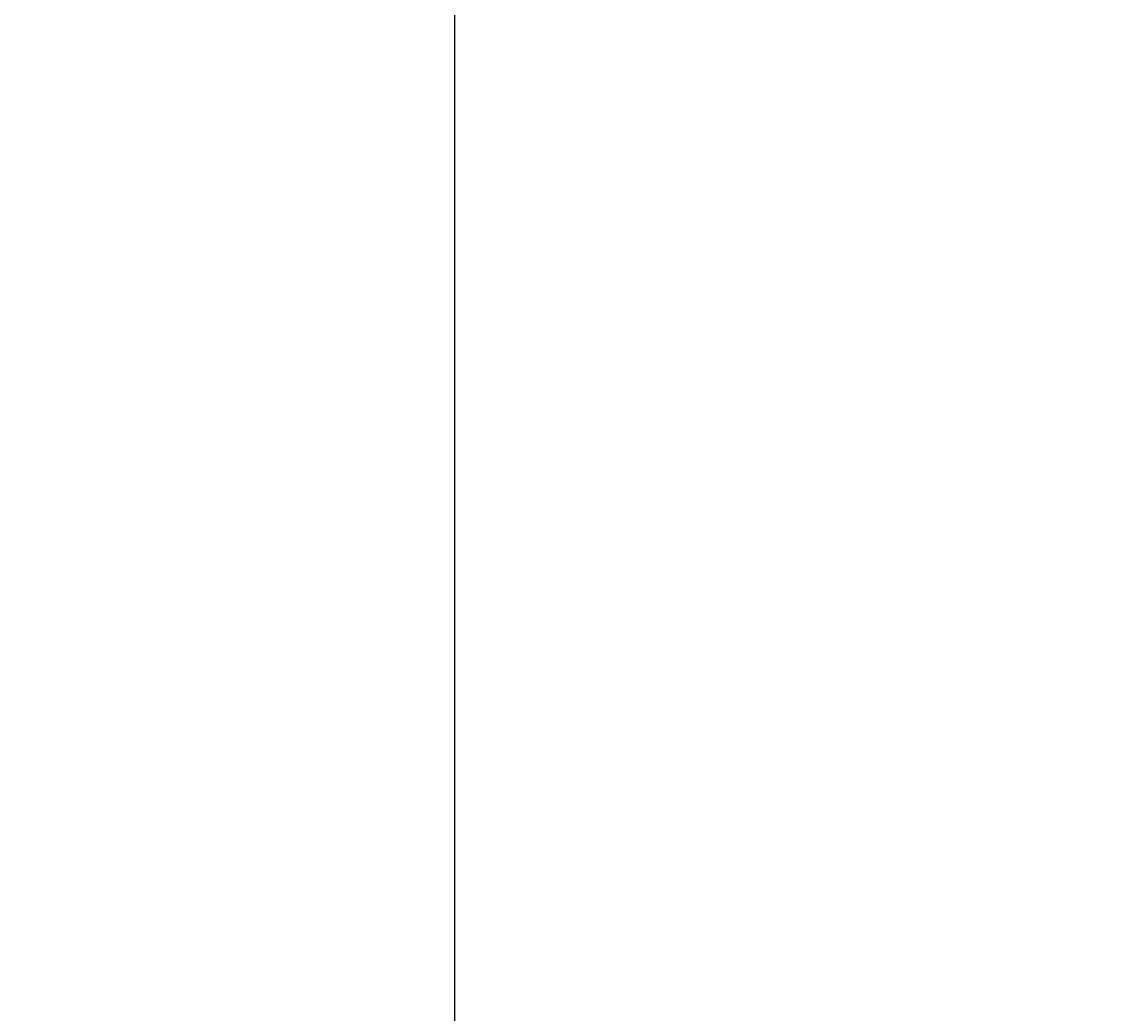
# Model space of a CAD drawing. Units: inches. Extents: x 1998 to 2588, y 1139 to 1977.
# Tile 83 of 134: x 2397 to 2425, y 1427 to 1452. Entities that reach past the tile are written whole.
import ezdxf

# ---------------------------------------------------------------- set-up
doc = ezdxf.new("R2010")
doc.units = ezdxf.units.IN
doc.layers.add('A-ANNO-DIMS', color=2, linetype='Continuous', lineweight=18)
doc.styles.get("Standard").update_dxf_attribs({"font": 'arial.ttf'})
doc.dimstyles.get("Standard").update_dxf_attribs({"dimtxt": 0.18, "dimasz": 0.18, "dimexe": 0.18, "dimexo": 0.0625, "dimgap": 0.09, "dimtad": 0, "dimtih": 1, "dimtoh": 1, "dimdec": 4, "dimzin": 0, "dimdsep": 46, "dimtxsty": 'Standard', "dimcen": 0.09, "dimadec": 0, "dimazin": 0, "dimtfac": 1, "dimtdec": 4, "dimtofl": 0, "dimtmove": 0, "dimatfit": 3, "dimfxl": 1, "dimtolj": 1, "dimtzin": 0, "dimarcsym": 0})

# ---------------------------------------------------------------- blocks, each defined once
blk = doc.blocks.new('*D23')
at = {"layer": 'A-ANNO-DIMS', "color": 0, "lineweight": -2, "transparency": 16777216}
for p, q in [((2549.179, 1476.17), (2549.179, 1138.602)), ((2059.473, 1413.17), (2059.473, 1138.602)), ((2059.653, 1138.782), (2303.928, 1138.782)), ((2548.999, 1138.782), (2304.723, 1138.782))]:
    blk.add_line(p, q, dxfattribs=at)
at = {"layer": 'A-ANNO-DIMS', "color": 0, "transparency": 16777216}
for points in [[(2059.653, 1138.812), (2059.653, 1138.752), (2059.473, 1138.782)], [(2548.999, 1138.812), (2548.999, 1138.752), (2549.179, 1138.782)]]:
    blk.add_solid(points, dxfattribs=at)
at = {"layer": 'Defpoints', "color": 0, "transparency": 16777216}
for p in [(2549.179, 1476.232), (2059.473, 1413.232), (2549.179, 1138.782)]:
    blk.add_point(p, dxfattribs=at)
at = {"layer": 'A-ANNO-DIMS', "color": 0, "transparency": 16777216, "insert": (2304.326, 1138.782), "char_height": 0.18, "attachment_point": 5}
blk.add_mtext('\\A1;489.7', dxfattribs=at)
blk = doc.blocks.new('*D24')
at = {"layer": 'A-ANNO-DIMS', "color": 0, "lineweight": -2, "transparency": 16777216}
for p, q in [((2398.535, 1911.232), (2588.309, 1911.232)), ((2588.129, 1911.052), (2588.129, 1570.164)), ((2588.129, 1228.912), (2588.129, 1569.8)), ((2527.535, 1228.732), (2588.309, 1228.732))]:
    blk.add_line(p, q, dxfattribs=at)
at = {"layer": 'A-ANNO-DIMS', "color": 0, "transparency": 16777216}
for points in [[(2588.099, 1911.052), (2588.159, 1911.052), (2588.129, 1911.232)], [(2588.099, 1228.912), (2588.159, 1228.912), (2588.129, 1228.732)]]:
    blk.add_solid(points, dxfattribs=at)
at = {"layer": 'Defpoints', "color": 0, "transparency": 16777216}
for p in [(2398.473, 1911.232), (2588.129, 1911.232), (2527.473, 1228.732)]:
    blk.add_point(p, dxfattribs=at)
at = {"layer": 'A-ANNO-DIMS', "color": 0, "transparency": 16777216, "insert": (2588.129, 1569.982), "char_height": 0.18, "attachment_point": 5}
blk.add_mtext('\\A1;682.5', dxfattribs=at)
blk = doc.blocks.new('*D33')
at = {"layer": 'A-ANNO-DIMS', "color": 0, "lineweight": -2, "transparency": 16777216}
for p, q in [((2407.973, 1480.67), (2407.973, 1138.602)), ((2498.179, 1480.67), (2498.179, 1138.602)), ((2408.153, 1138.782), (2452.753, 1138.782)), ((2497.999, 1138.782), (2453.399, 1138.782))]:
    blk.add_line(p, q, dxfattribs=at)
at = {"layer": 'A-ANNO-DIMS', "color": 0, "transparency": 16777216}
for points in [[(2408.153, 1138.812), (2408.153, 1138.752), (2407.973, 1138.782)], [(2497.999, 1138.812), (2497.999, 1138.752), (2498.179, 1138.782)]]:
    blk.add_solid(points, dxfattribs=at)
at = {"layer": 'Defpoints', "color": 0, "transparency": 16777216}
for p in [(2407.973, 1480.732), (2498.179, 1480.732), (2498.179, 1138.782)]:
    blk.add_point(p, dxfattribs=at)
at = {"layer": 'A-ANNO-DIMS', "color": 0, "transparency": 16777216, "insert": (2453.076, 1138.782), "char_height": 0.18, "attachment_point": 5}
blk.add_mtext('\\A1;90.2', dxfattribs=at)
blk = doc.blocks.new('*D43')
at = {"layer": 'A-ANNO-DIMS', "color": 0, "lineweight": -2, "transparency": 16777216}
for p, q in [((2407.973, 1594.67), (2407.973, 1138.602)), ((2345.973, 1588.67), (2345.973, 1138.602)), ((2346.153, 1138.782), (2376.754, 1138.782)), ((2407.793, 1138.782), (2377.191, 1138.782))]:
    blk.add_line(p, q, dxfattribs=at)
at = {"layer": 'A-ANNO-DIMS', "color": 0, "transparency": 16777216}
for points in [[(2346.153, 1138.812), (2346.153, 1138.752), (2345.973, 1138.782)], [(2407.793, 1138.812), (2407.793, 1138.752), (2407.973, 1138.782)]]:
    blk.add_solid(points, dxfattribs=at)
at = {"layer": 'Defpoints', "color": 0, "transparency": 16777216}
for p in [(2407.973, 1594.732), (2345.973, 1588.732), (2407.973, 1138.782)]:
    blk.add_point(p, dxfattribs=at)
at = {"layer": 'A-ANNO-DIMS', "color": 0, "transparency": 16777216, "insert": (2376.973, 1138.782), "char_height": 0.18, "attachment_point": 5}
blk.add_mtext('\\A1;62', dxfattribs=at)

msp = doc.modelspace()

# ---------------------------------------------------------------- dimensions: what is measured, and where the dimension line sits
at = {"layer": 'A-ANNO-DIMS'}
dim = msp.add_linear_dim(base=(2588.1286, 1911.2324), p1=(2527.4729, 1228.7324), p2=(2398.4729, 1911.2324), angle=90, dimstyle='Standard', override={"dimdec": 1, "dimlfac": 1, "dimrnd": 0, "dimzin": 0, "dimdsep": 46, "dimlunit": 2}, dxfattribs=at)
dim.commit()
dim.dimension.update_dxf_attribs({"geometry": '*D24', "text_midpoint": (2588.1286, 1569.9824)})
for base, p1, p2, override, picture, middle in [((2407.9729, 1138.7824), (2345.9729, 1588.7324), (2407.9729, 1594.7324), {"dimdec": 0, "dimlfac": 1, "dimrnd": 0, "dimzin": 0, "dimdsep": 46, "dimlunit": 2}, '*D43', (2376.9729, 1138.7824)), ((2498.1786, 1138.7824), (2407.9729, 1480.7324), (2498.1786, 1480.7324), {"dimdec": 1, "dimlfac": 1, "dimrnd": 0, "dimzin": 0, "dimdsep": 46, "dimlunit": 2}, '*D33', (2453.0757, 1138.7824)), ((2549.1786, 1138.7824), (2059.4729, 1413.2324), (2549.1786, 1476.2324), {"dimdec": 1, "dimlfac": 1, "dimrnd": 0, "dimzin": 0, "dimdsep": 46, "dimlunit": 2}, '*D23', (2304.3257, 1138.7824))]:
    dim = msp.add_linear_dim(base=base, p1=p1, p2=p2, dimstyle='Standard', override=override, dxfattribs=at)
    dim.commit()
    dim.dimension.update_dxf_attribs({"geometry": picture, "text_midpoint": middle})

doc.saveas('drawing.dxf')
